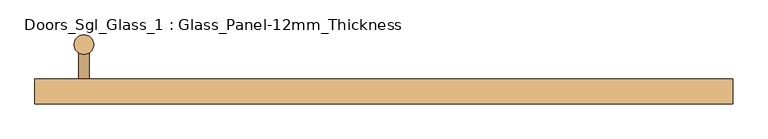
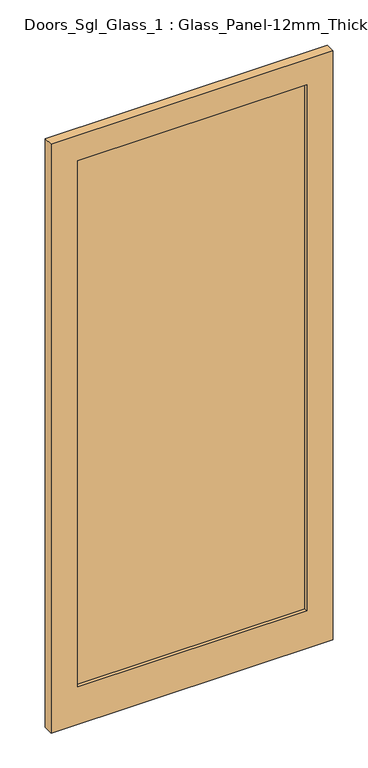
"""IFC4 building model written with IfcOpenShell, lengths in millimetres: door geometry, Doors_Sgl_Glass_1 : Glass_Panel-12mm_Thickness."""

from ifc_helpers import new_model, si_unit, point, frame, frame_2d, origin, place, context, project, spatial, polyline, circle_curve, trimmed, segment, composite_curve, outline, extrude, source, transform, mapped, element, save


def doors_sgl_glass_1_glass_panel_12mm_thickness_f5485519(model_context):
    return source(origin(), model_context, "Body", "SweptSolid", [
        extrude(outline(polyline([(434.314808, 50.0), (434.314808, 38.0), (-434.314808, 38.0), (-434.314808, 50.0), (434.314808, 50.0)])), frame((0.0, 0.0, 150.0), z_axis=(0.0, 0.0, 1.0), x_axis=(1.0, 0.0, 0.0)), (0.0, 0.0, 1.0), 2105.0),
        extrude(outline(polyline([(0.0, -534.314808), (0.0, 534.314808), (2355.0, 534.314808), (2355.0, -534.314808), (0.0, -534.314808)]), holes=[polyline([(2255.0, 434.314808), (150.0, 434.314808), (150.0, -434.314808), (2255.0, -434.314808), (2255.0, 434.314808)])]), frame((0.0, 25.0, 0.0), z_axis=(0.0, 1.0, 0.0), x_axis=(0.0, 0.0, 1.0)), (0.0, 0.0, 1.0), 38.0),
        extrude(outline(composite_curve([segment(trimmed(circle_curve(frame_2d((1450.0, -459.314808)), 8.0), [point((1450.0, -451.314808))], [point((1450.0, -467.314808))], False, "CARTESIAN"), True, "CONTINUOUS"), segment(trimmed(circle_curve(frame_2d((1450.0, -459.314808)), 8.0), [point((1450.0, -467.314808))], [point((1450.0, -451.314808))], False, "CARTESIAN"), True, "CONTINUOUS")], self_intersect=False)), frame((0.0, 63.0, 0.0), z_axis=(0.0, 1.0, 0.0), x_axis=(0.0, 0.0, 1.0)), (0.0, 0.0, 1.0), 53.0),
        extrude(outline(composite_curve([segment(trimmed(circle_curve(frame_2d((750.0, -459.314808)), 8.0), [point((750.0, -451.314808))], [point((750.0, -467.314808))], False, "CARTESIAN"), True, "CONTINUOUS"), segment(trimmed(circle_curve(frame_2d((750.0, -459.314808)), 8.0), [point((750.0, -467.314808))], [point((750.0, -451.314808))], False, "CARTESIAN"), True, "CONTINUOUS")], self_intersect=False)), frame((0.0, 63.0, 0.0), z_axis=(0.0, 1.0, 0.0), x_axis=(0.0, 0.0, 1.0)), (0.0, 0.0, 1.0), 53.0),
        extrude(outline(composite_curve([segment(trimmed(circle_curve(frame_2d((-459.314808, 116.0)), 15.0), [point((-459.314808, 101.0))], [point((-459.314808, 131.0))], False, "CARTESIAN"), True, "CONTINUOUS"), segment(trimmed(circle_curve(frame_2d((-459.314808, 116.0)), 15.0), [point((-459.314808, 131.0))], [point((-459.314808, 101.0))], False, "CARTESIAN"), True, "CONTINUOUS")], self_intersect=False)), frame((0.0, 0.0, 650.0), z_axis=(0.0, 0.0, 1.0), x_axis=(1.0, 0.0, 0.0)), (0.0, 0.0, 1.0), 900.0),
    ])


if __name__ == "__main__":
    model = new_model("IFC4")
    model_context = context("Model", 3, world=origin())
    ifc_project = project(units=[si_unit("LENGTHUNIT", "METRE", prefix="MILLI")], contexts=[model_context])
    site = spatial("IfcSite", under=ifc_project)
    building = spatial("IfcBuilding", under=site)
    placement = place(None, origin())
    doors_sgl_glass_1_glass_panel_12mm_thickness_shape = doors_sgl_glass_1_glass_panel_12mm_thickness_f5485519(model_context)
    element("IfcDoor", 1, ObjectType="Doors_Sgl_Glass_1 : Glass_Panel-12mm_Thickness", at=placement, inside=building, context=model_context, shape_type="MappedRepresentation", body=[
        mapped(doors_sgl_glass_1_glass_panel_12mm_thickness_shape, transform((0.0, 0.0, 0.0), x_axis=(1.0, 0.0, 0.0), y_axis=(0.0, 1.0, 0.0), z_axis=(0.0, 0.0, 1.0))),
    ])
    save(model, "model.ifc")

# Revit data of these elements
# Type "Doors_Sgl_Glass_1 : Glass_Panel-12mm_Thickness"
#   Type Mark = "60"
#   Construction Type Id = "GSP4R"
#   Keynote = "H11"
#   Analytic Construction = "1/8 in Pilkington single glazing"
#   Visual Light Transmittance = 0.9
#   Stile Top Rail = 0' - 3.93701"
#   Stile Shutting = 0' - 3.93701"
#   Stile Hanging = 0' - 3.93701"
#   Stile Bottom Rail = 0' - 5.90551"
#   Solar Heat Gain Coefficient = 0.78
#   Offset = 0' - 1.9685"
#   Heat Transfer Coefficient (U) = 3.6886 W/(m²·K)
#   Handle X Distance = 0' - 2.95276"
#   Glazing Thickness = 0' - 0.47244"
#   Define Thermal Properties by = 1
#   Material Ironmongery = Metal - Aluminum
#   Material Frame = Metal - Aluminum
#   Material Glass = Glass
#   Function = (empty or 0)
# Element 1 (IfcDoor, "Doors_Sgl_Glass_1 : Glass_Panel-12mm_Thickness")
#   Materials on its faces: "Metal - Aluminum", "Glass"
# Materials
#   "Metal - Aluminum": class "Metal", colour RGB 247 247 247, transparency 0
#   "Glass": class "Glass", colour RGB 0 128 192, transparency 0.9, Description = "Soda Lime Glass", Cost = 0
